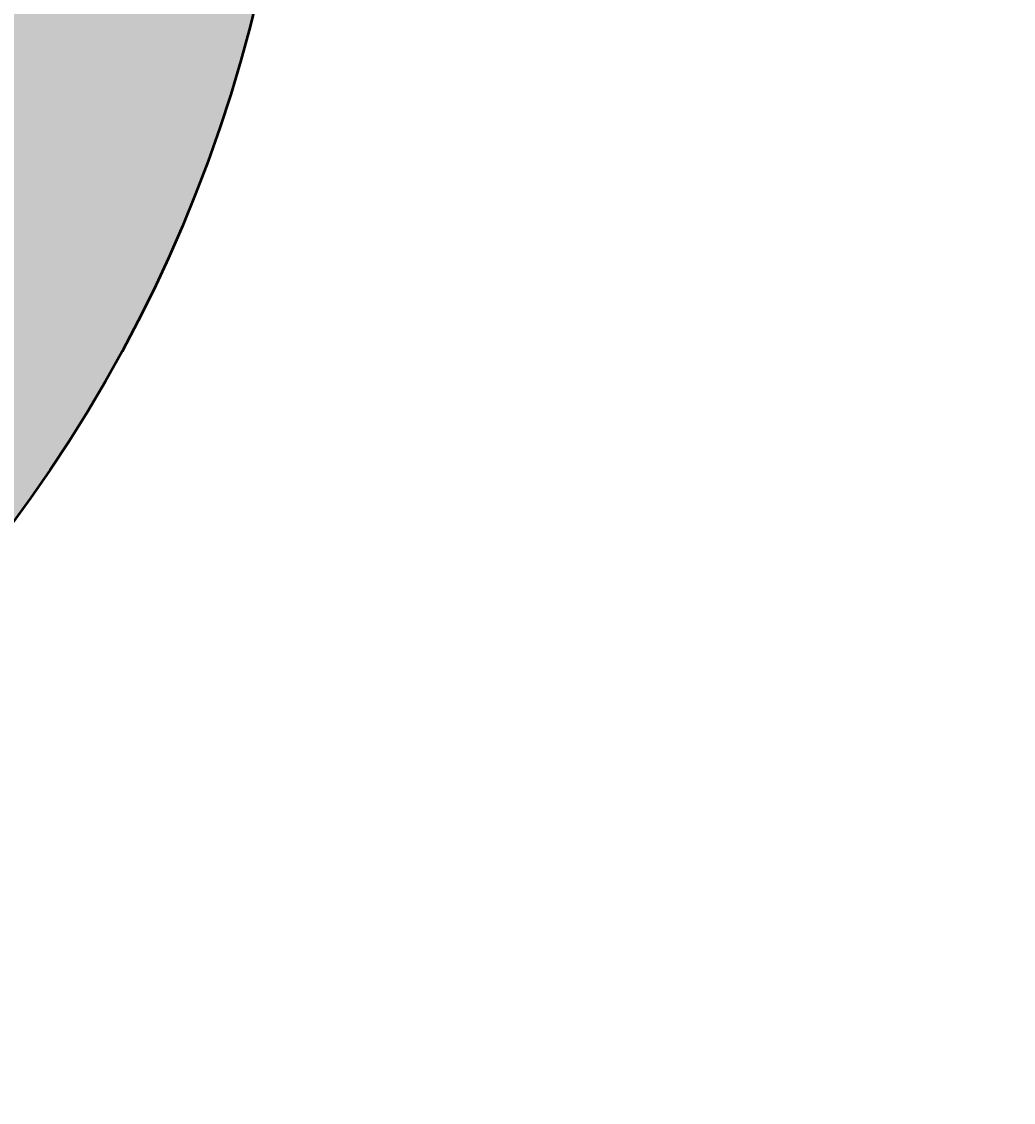
# Model space of a CAD drawing. Units: inches. Extents: x 139261 to 139415, y 52839 to 52963.
# Tile 12 of 20: x 139381 to 139415, y 52850 to 52888. Entities that reach past the tile are written whole.
import ezdxf

# ---------------------------------------------------------------- set-up
doc = ezdxf.new("R2010")
doc.units = ezdxf.units.IN
doc.header["$MEASUREMENT"] = 0
for name, color, linetype, lineweight in [('M-DIMS', 2, 'Continuous', 25), ('M-HATC', 8, 'Continuous', 18), ('M-OUTL', 7, 'Continuous', 50)]:
    doc.layers.add(name, color=color, linetype=linetype, lineweight=lineweight)
doc.styles.get("Standard").update_dxf_attribs({"font": 'arial.ttf'})
doc.dimstyles.get("Standard").update_dxf_attribs({"dimtxt": 0.18, "dimasz": 0.18, "dimexe": 0.18, "dimexo": 0.0625, "dimgap": 0.09, "dimtad": 0, "dimtih": 1, "dimtoh": 1, "dimdec": 4, "dimzin": 0, "dimdsep": 46, "dimtxsty": 'Standard', "dimcen": 0.09, "dimadec": 0, "dimazin": 0, "dimtfac": 1, "dimtdec": 4, "dimtofl": 0, "dimtmove": 0, "dimatfit": 3, "dimfxl": 1, "dimtolj": 1, "dimtzin": 0, "dimarcsym": 0})

# ---------------------------------------------------------------- blocks, each defined once
blk = doc.blocks.new('*D4')
at = {"layer": 'Defpoints', "color": 0, "transparency": 16777216}
for p in [(139373.053, 52923.26), (139307.661, 52877.175)]:
    blk.add_point(p, dxfattribs=at)
at = {"layer": 'M-DIMS', "color": 0, "lineweight": -2, "transparency": 16777216}
for p, q in [((139414.011, 52952.126), (139373.2, 52923.364)), ((139414.191, 52952.126), (139414.011, 52952.126)), ((139340.267, 52900.217), (139340.447, 52900.217)), ((139340.357, 52900.127), (139340.357, 52900.307))]:
    blk.add_line(p, q, dxfattribs=at)
blk.add_arc((139340.357, 52900.217), 40, 34.9168, 52.0771, dxfattribs=at)
at = {"layer": 'M-DIMS', "color": 0, "transparency": 16777216}
blk.add_solid([(139373.183, 52923.388), (139373.217, 52923.339), (139373.053, 52923.26)], dxfattribs=at)
at = {"layer": 'M-DIMS', "color": 0, "transparency": 16777216, "insert": (139414.822, 52952.126), "char_height": 0.18, "attachment_point": 5}
blk.add_mtext('\\A1;∅80.0000', dxfattribs=at)

msp = doc.modelspace()

# ---------------------------------------------------------------- hatches: boundary and pattern name
at = {"layer": 'M-HATC'}
h = msp.add_hatch(color=256, dxfattribs=at)
h.dxf.hatch_style = 1
h.paths.add_polyline_path([(139290.35689, 52900.21749, 1), (139390.35689, 52900.21749, 1)])
h.paths.add_polyline_path([(139335.36666, 52939.90499, -0.01563646), (139335.35689, 52940.21749, -1), (139345.35689, 52940.21749, -0.01563646), (139345.34711, 52939.90499, -0.13461315), (139364.89157, 52931.80941, -0.691035), (139373.64116, 52928.50176, -0.21521822), (139371.94881, 52924.75216, -0.13461315), (139380.04439, 52905.20771, -0.43265224), (139385.35689, 52900.21749, -0.43265224), (139380.04439, 52895.22726, -0.13461315), (139371.94881, 52875.68281, -0.21521822), (139373.64116, 52871.93321, -0.691035), (139364.89157, 52868.62556, -0.13461315), (139345.34711, 52860.52999, -0.01563646), (139345.35689, 52860.21749, -1), (139335.35689, 52860.21749, -0.01563646), (139335.36666, 52860.52999, -0.13461315), (139315.82221, 52868.62556, -0.691035), (139307.07262, 52871.93321, -0.21521822), (139308.76496, 52875.68281, -0.13461315), (139300.66939, 52895.22726, -0.43265224), (139295.35689, 52900.21749, -0.43265224), (139300.66939, 52905.20771, -0.13461315), (139308.76496, 52924.75216, -0.21521822), (139307.07262, 52928.50176, -0.691035), (139315.82221, 52931.80941, -0.13461315)], flags=16)
h.paths.add_polyline_path([(139365.35689, 52900.21749, -1), (139315.35689, 52900.21749, -1)], flags=0)
h.paths.add_polyline_path([(139323.71474, 52911.30978), (139356.99903, 52911.30978, -0.3027197), (139356.99903, 52889.12519), (139323.71474, 52889.12519, -0.3027197)], flags=0)
h.paths.add_polyline_path([(139364.89157, 52931.80941, 0.13461315), (139345.34711, 52939.90499, -0.93933644), (139335.36666, 52939.90499, 0.13461315), (139315.82221, 52931.80941, -0.18270763), (139317.07262, 52928.50176, -0.64579494), (139308.76496, 52924.75216, 0.13461315), (139300.66939, 52905.20771, -0.39601219), (139305.35689, 52900.21749, -0.39601219), (139300.66939, 52895.22726, 0.13461315), (139308.76496, 52875.68281, -0.64579494), (139317.07262, 52871.93321, -0.18270763), (139315.82221, 52868.62556, 0.13461315), (139335.36666, 52860.52999, -0.93933644), (139345.34711, 52860.52999, 0.13461315), (139364.89157, 52868.62556, -0.18270763), (139363.64116, 52871.93321, -0.64579494), (139371.94881, 52875.68281, 0.13461315), (139380.04439, 52895.22726, -0.39601219), (139375.35689, 52900.21749, -0.39601219), (139380.04439, 52905.20771, 0.13461315), (139371.94881, 52924.75216, -0.64579494), (139363.64116, 52928.50176, -0.18270763)], flags=0)

# ---------------------------------------------------------------- linework, layer by layer
at = {"layer": 'M-OUTL'}
msp.add_circle((139340.35689, 52900.21749), 50, dxfattribs=at)

# ---------------------------------------------------------------- dimensions: what is measured, and where the dimension line sits
at = {"layer": 'M-DIMS'}
dim = msp.add_diameter_dim_2p(p1=(139307.66087, 52877.17469), p2=(139373.0529, 52923.26028), dimstyle='Standard', override={"dimclrd": 0, "dimclre": 0, "dimclrt": 0}, dxfattribs=at)
dim.commit()
dim.dimension.update_dxf_attribs({"geometry": '*D4', "text_midpoint": (139414.82217, 52952.12585), "dimtype": 163})

doc.saveas('drawing.dxf')
